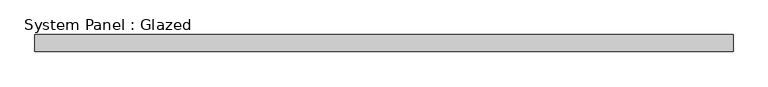
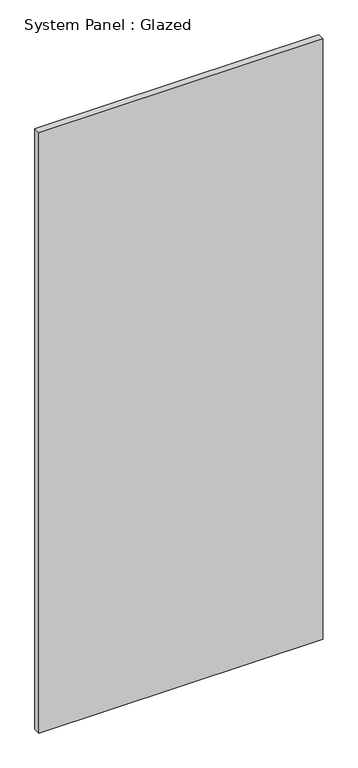
"""IFC4 building model written with IfcOpenShell, lengths in millimetres: plate geometry, System Panel : Glazed."""

from ifc_helpers import new_model, si_unit, origin, origin_with_axes, place, context, project, spatial, polyline, outline, extrude, source, transform, mapped, element, save


def system_panel_glazed_cc935e45(model_context):
    return source(origin(), model_context, "Body", "SweptSolid", [
        extrude(outline(polyline([(523.875, 19.05), (-523.875, 19.05), (-523.875, 44.45), (523.875, 44.45), (523.875, 19.05)])), origin_with_axes(), (0.0, 0.0, 1.0), 2343.15),
    ])


if __name__ == "__main__":
    model = new_model("IFC4")
    model_context = context("Model", 3, world=origin())
    ifc_project = project(units=[si_unit("LENGTHUNIT", "METRE", prefix="MILLI")], contexts=[model_context])
    site = spatial("IfcSite", under=ifc_project)
    building = spatial("IfcBuilding", under=site)
    placement = place(None, origin())
    system_panel_glazed_shape = system_panel_glazed_cc935e45(model_context)
    element("IfcPlate", 1, ObjectType="System Panel : Glazed", at=placement, inside=building, context=model_context, shape_type="MappedRepresentation", body=[
        mapped(system_panel_glazed_shape, transform((0.0, 0.0, 0.0), x_axis=(1.0, 0.0, 0.0), y_axis=(0.0, 1.0, 0.0), z_axis=(0.0, 0.0, 1.0))),
    ])
    save(model, "model.ifc")

# Revit data of these elements
# Type "System Panel : Glazed"
#   Construction Type Id = "GSP4R"
#   Analytic Construction = "1/8 in Pilkington single glazing"
#   Visual Light Transmittance = 0.9
#   Solar Heat Gain Coefficient = 0.86
#   Heat Transfer Coefficient (U) = 1.18115 BTU/(h·ft²·°F)
#   Define Thermal Properties by = 1
# Element 1 (IfcPlate, "System Panel : Glazed")
#   Materials on its faces: "Glass"
# Materials
#   "Glass": class "Glass", colour RGB 0 128 192, transparency 0.75, Description = "Soda Lime Glass", Cost = 0
